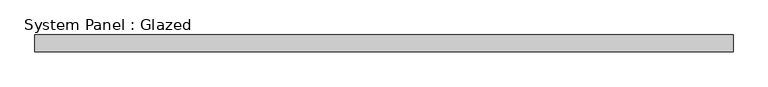
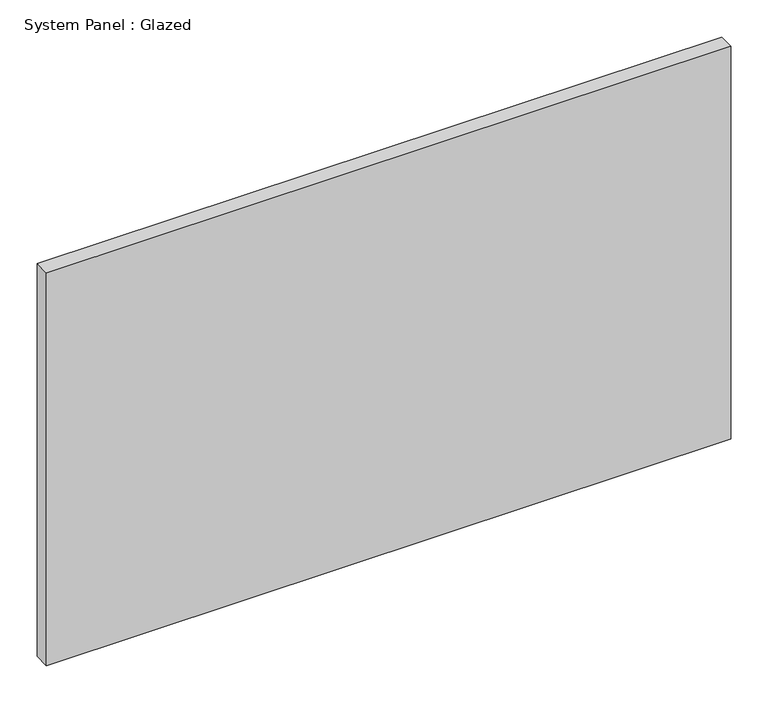
"""IFC4 building model written with IfcOpenShell, lengths in millimetres: plate geometry, System Panel : Glazed."""

from ifc_helpers import new_model, si_unit, origin, origin_with_axes, place, context, project, spatial, polyline, outline, extrude, source, transform, mapped, element, save


def system_panel_glazed_0a58f99c(model_context):
    return source(origin(), model_context, "Body", "SweptSolid", [
        extrude(outline(polyline([(533.532314, 19.05), (-533.532314, 19.05), (-533.532314, 44.45), (533.532314, 44.45), (533.532314, 19.05)])), origin_with_axes(), (0.0, 0.0, 1.0), 647.7),
    ])


if __name__ == "__main__":
    model = new_model("IFC4")
    model_context = context("Model", 3, world=origin())
    ifc_project = project(units=[si_unit("LENGTHUNIT", "METRE", prefix="MILLI")], contexts=[model_context])
    site = spatial("IfcSite", under=ifc_project)
    building = spatial("IfcBuilding", under=site)
    placement = place(None, origin())
    system_panel_glazed_shape = system_panel_glazed_0a58f99c(model_context)
    element("IfcPlate", 1, ObjectType="System Panel : Glazed", at=placement, inside=building, context=model_context, shape_type="MappedRepresentation", body=[
        mapped(system_panel_glazed_shape, transform((0.0, 0.0, 0.0), x_axis=(1.0, 0.0, 0.0), y_axis=(0.0, 1.0, 0.0), z_axis=(0.0, 0.0, 1.0))),
    ])
    save(model, "model.ifc")

# Revit data of these elements
# Type "System Panel : Glazed"
#   Construction Type Id = "GSP4R"
#   Analytic Construction = "1/8 in Pilkington single glazing"
#   Visual Light Transmittance = 0.9
#   Solar Heat Gain Coefficient = 0.86
#   Heat Transfer Coefficient (U) = 1.18115 BTU/(h·ft²·°F)
#   Define Thermal Properties by = 1
# Element 1 (IfcPlate, "System Panel : Glazed")
#   Materials on its faces: "Glass"
# Materials
#   "Glass": class "Glass", colour RGB 0 128 192, transparency 0.75, Description = "Soda Lime Glass", Cost = 0
